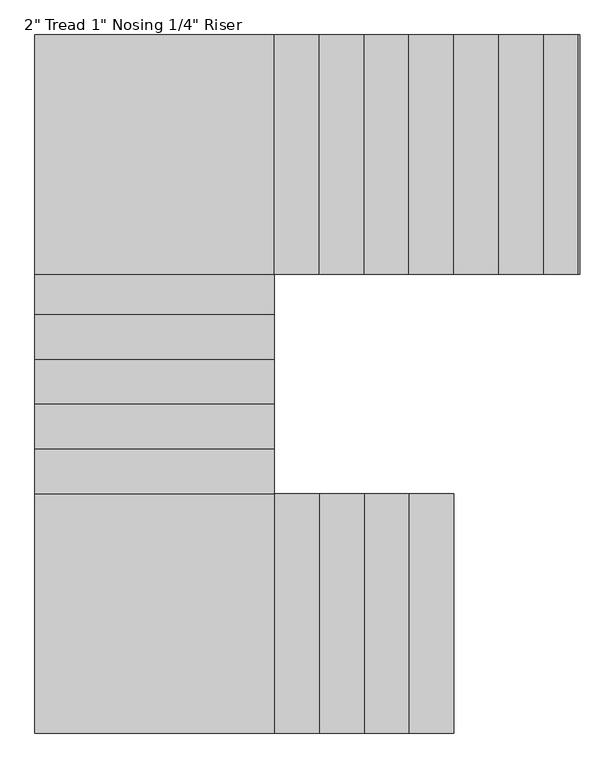
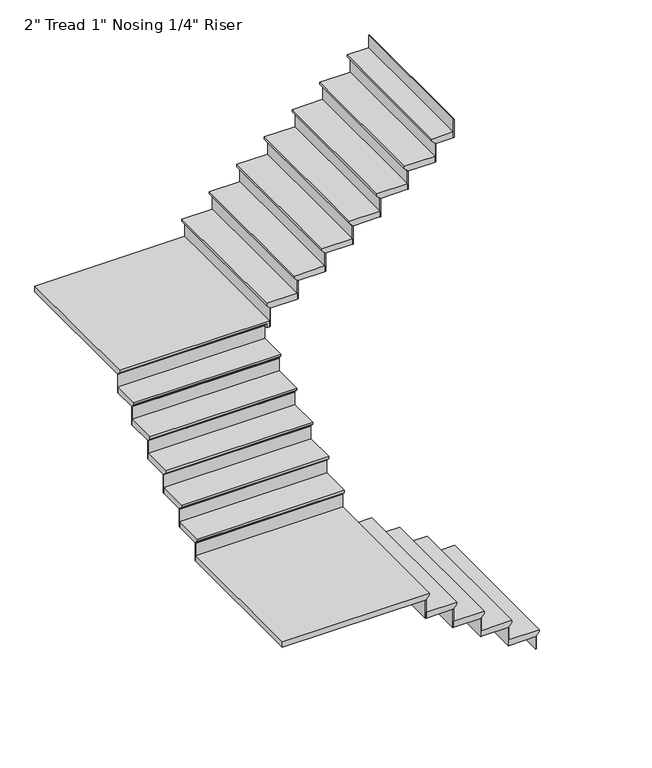
"""IFC4 building model written with IfcOpenShell, lengths in millimetres: stair flight geometry."""

from ifc_helpers import new_model, si_unit, origin, place, context, project, spatial, faceted_brep, source, transform, mapped, element, save


def stair_flight_424eac51(model_context):
    return source(origin(), model_context, "Body", "Brep", [
        faceted_brep([(-2683.1105391, -1521.8373761, 6389.7710526), (-2683.1105391, -1521.8373761, 6408.8210526), (-2683.1105391, -2741.0373761, 6408.8210526), (-2683.1105391, -2741.0373761, 6389.7710526), (-2708.5105391, -1521.8373761, 6364.3710526), (-2708.5105391, -2741.0373761, 6364.3710526), (-2937.1105391, -1521.8373761, 6408.8210526), (-2937.1105391, -2741.0373761, 6408.8210526), (-2708.5105391, -2741.0373761, 6358.0210526), (-2937.1105391, -2741.0373761, 6358.0210526), (-2937.1105391, -1521.8373761, 6358.0210526), (-2708.5105391, -1521.8373761, 6358.0210526)], [[[0, 1, 2, 3]], [[4, 0, 3, 5]], [[2, 1, 6, 7]], [[8, 9, 10, 11]], [[2, 7, 9, 8, 5, 3]], [[8, 11, 4, 5]], [[6, 1, 0, 4, 11, 10]], [[7, 6, 10, 9]]]),
        faceted_brep([(-2708.5105391, -1521.8373761, 6358.0210526), (-2708.5105391, -1521.8373761, 6248.4), (-2714.8605391, -1521.8373761, 6248.4), (-2714.8605391, -1521.8373761, 6358.0210526), (-2708.5105391, -2741.0373761, 6358.0210526), (-2714.8605391, -2741.0373761, 6358.0210526), (-2714.8605391, -2741.0373761, 6248.4), (-2708.5105391, -2741.0373761, 6248.4)], [[[0, 1, 2, 3]], [[4, 5, 6, 7]], [[1, 0, 4, 7]], [[2, 1, 7, 6]], [[3, 2, 6, 5]], [[0, 3, 5, 4]]]),
        faceted_brep([(-2937.1105391, -1521.8373761, 6518.4421053), (-2937.1105391, -1521.8373761, 6358.0210526), (-2943.4605391, -1521.8373761, 6358.0210526), (-2943.4605391, -1521.8373761, 6518.4421053), (-2937.1105391, -2741.0373761, 6518.4421053), (-2943.4605391, -2741.0373761, 6518.4421053), (-2943.4605391, -2741.0373761, 6358.0210526), (-2937.1105391, -2741.0373761, 6358.0210526)], [[[0, 1, 2, 3]], [[4, 5, 6, 7]], [[1, 0, 4, 7]], [[2, 1, 7, 6]], [[3, 2, 6, 5]], [[0, 3, 5, 4]]]),
        faceted_brep([(-2911.7105391, -2741.0373761, 6569.2421053), (-2911.7105391, -1521.8373761, 6569.2421053), (-3165.7105391, -1521.8373761, 6569.2421053), (-3165.7105391, -2741.0373761, 6569.2421053), (-2937.1105391, -2741.0373761, 6518.4421053), (-3165.7105391, -2741.0373761, 6518.4421053), (-3165.7105391, -1521.8373761, 6518.4421053), (-2937.1105391, -1521.8373761, 6518.4421053), (-2937.1105391, -2741.0373761, 6524.7921053), (-2911.7105391, -2741.0373761, 6550.1921053), (-2937.1105391, -1521.8373761, 6524.7921053), (-2911.7105391, -1521.8373761, 6550.1921053)], [[[0, 1, 2, 3]], [[4, 5, 6, 7]], [[0, 3, 5, 4, 8, 9]], [[4, 7, 10, 8]], [[2, 1, 11, 10, 7, 6]], [[3, 2, 6, 5]], [[11, 1, 0, 9]], [[10, 11, 9, 8]]]),
        faceted_brep([(-3165.7105391, -1521.8373761, 6678.8631579), (-3165.7105391, -1521.8373761, 6518.4421053), (-3172.0605391, -1521.8373761, 6518.4421053), (-3172.0605391, -1521.8373761, 6678.8631579), (-3165.7105391, -2741.0373761, 6678.8631579), (-3172.0605391, -2741.0373761, 6678.8631579), (-3172.0605391, -2741.0373761, 6518.4421053), (-3165.7105391, -2741.0373761, 6518.4421053)], [[[0, 1, 2, 3]], [[4, 5, 6, 7]], [[1, 0, 4, 7]], [[2, 1, 7, 6]], [[3, 2, 6, 5]], [[0, 3, 5, 4]]]),
        faceted_brep([(-3140.3105391, -2741.0373761, 6729.6631579), (-3140.3105391, -1521.8373761, 6729.6631579), (-3394.3105391, -1521.8373761, 6729.6631579), (-3394.3105391, -2741.0373761, 6729.6631579), (-3165.7105391, -2741.0373761, 6678.8631579), (-3394.3105391, -2741.0373761, 6678.8631579), (-3394.3105391, -1521.8373761, 6678.8631579), (-3165.7105391, -1521.8373761, 6678.8631579), (-3165.7105391, -2741.0373761, 6685.2131579), (-3140.3105391, -2741.0373761, 6710.6131579), (-3165.7105391, -1521.8373761, 6685.2131579), (-3140.3105391, -1521.8373761, 6710.6131579)], [[[0, 1, 2, 3]], [[4, 5, 6, 7]], [[0, 3, 5, 4, 8, 9]], [[4, 7, 10, 8]], [[2, 1, 11, 10, 7, 6]], [[3, 2, 6, 5]], [[11, 1, 0, 9]], [[10, 11, 9, 8]]]),
        faceted_brep([(-3394.3105391, -1521.8373761, 6839.2842105), (-3394.3105391, -1521.8373761, 6678.8631579), (-3400.6605391, -1521.8373761, 6678.8631579), (-3400.6605391, -1521.8373761, 6839.2842105), (-3394.3105391, -2741.0373761, 6839.2842105), (-3400.6605391, -2741.0373761, 6839.2842105), (-3400.6605391, -2741.0373761, 6678.8631579), (-3394.3105391, -2741.0373761, 6678.8631579)], [[[0, 1, 2, 3]], [[4, 5, 6, 7]], [[1, 0, 4, 7]], [[2, 1, 7, 6]], [[3, 2, 6, 5]], [[0, 3, 5, 4]]]),
        faceted_brep([(-3368.9105391, -2741.0373761, 6890.0842105), (-3368.9105391, -1521.8373761, 6890.0842105), (-3622.9105391, -1521.8373761, 6890.0842105), (-3622.9105391, -2741.0373761, 6890.0842105), (-3394.3105391, -2741.0373761, 6839.2842105), (-3622.9105391, -2741.0373761, 6839.2842105), (-3622.9105391, -1521.8373761, 6839.2842105), (-3394.3105391, -1521.8373761, 6839.2842105), (-3394.3105391, -2741.0373761, 6845.6342105), (-3368.9105391, -2741.0373761, 6871.0342105), (-3394.3105391, -1521.8373761, 6845.6342105), (-3368.9105391, -1521.8373761, 6871.0342105)], [[[0, 1, 2, 3]], [[4, 5, 6, 7]], [[0, 3, 5, 4, 8, 9]], [[4, 7, 10, 8]], [[2, 1, 11, 10, 7, 6]], [[3, 2, 6, 5]], [[11, 1, 0, 9]], [[10, 11, 9, 8]]]),
        faceted_brep([(-3622.9105391, -1521.8373761, 6999.7052632), (-3622.9105391, -1521.8373761, 6839.2842105), (-3629.2605391, -1521.8373761, 6839.2842105), (-3629.2605391, -1521.8373761, 6999.7052632), (-3622.9105391, -2741.0373761, 6999.7052632), (-3629.2605391, -2741.0373761, 6999.7052632), (-3629.2605391, -2741.0373761, 6839.2842105), (-3622.9105391, -2741.0373761, 6839.2842105)], [[[0, 1, 2, 3]], [[4, 5, 6, 7]], [[1, 0, 4, 7]], [[2, 1, 7, 6]], [[3, 2, 6, 5]], [[0, 3, 5, 4]]]),
        faceted_brep([(-4816.7105391, -1496.4373761, 7050.5052632), (-4816.7105391, -2741.0373761, 7050.5052632), (-3597.5105391, -2741.0373761, 7050.5052632), (-3597.5105391, -1496.4373761, 7050.5052632), (-4816.7105391, -2741.0373761, 6999.7052632), (-4816.7105391, -1496.4373761, 6999.7052632), (-3597.5105391, -1496.4373761, 6999.7052632), (-3597.5105391, -1521.8373761, 6999.7052632), (-3622.9105391, -1521.8373761, 6999.7052632), (-3622.9105391, -2741.0373761, 6999.7052632), (-3622.9105391, -2741.0373761, 7006.0552632), (-3597.5105391, -2741.0373761, 7031.4552632), (-3622.9105391, -1521.8373761, 7006.0552632), (-3597.5105391, -1521.8373761, 7031.4552632)], [[[0, 1, 2, 3]], [[4, 5, 6, 7, 8, 9]], [[1, 0, 5, 4]], [[2, 1, 4, 9, 10, 11]], [[9, 8, 12, 10]], [[8, 7, 13, 12]], [[3, 2, 11, 13, 7, 6]], [[0, 3, 6, 5]], [[11, 10, 12, 13]]]),
        faceted_brep([(-3597.5105391, -1496.4373761, 7160.1263158), (-3597.5105391, -1496.4373761, 6999.7052632), (-3597.5105391, -1490.0873761, 6999.7052632), (-3597.5105391, -1490.0873761, 7160.1263158), (-4816.7105391, -1496.4373761, 7160.1263158), (-4816.7105391, -1490.0873761, 7160.1263158), (-4816.7105391, -1490.0873761, 6999.7052632), (-4816.7105391, -1496.4373761, 6999.7052632)], [[[0, 1, 2, 3]], [[4, 5, 6, 7]], [[1, 0, 4, 7]], [[2, 1, 7, 6]], [[3, 2, 6, 5]], [[0, 3, 5, 4]]]),
        faceted_brep([(-4816.7105391, -1521.8373761, 7210.9263158), (-3597.5105391, -1521.8373761, 7210.9263158), (-3597.5105391, -1267.8373761, 7210.9263158), (-4816.7105391, -1267.8373761, 7210.9263158), (-4816.7105391, -1496.4373761, 7160.1263158), (-4816.7105391, -1267.8373761, 7160.1263158), (-3597.5105391, -1267.8373761, 7160.1263158), (-3597.5105391, -1496.4373761, 7160.1263158), (-4816.7105391, -1496.4373761, 7166.4763158), (-4816.7105391, -1521.8373761, 7191.8763158), (-3597.5105391, -1496.4373761, 7166.4763158), (-3597.5105391, -1521.8373761, 7191.8763158)], [[[0, 1, 2, 3]], [[4, 5, 6, 7]], [[0, 3, 5, 4, 8, 9]], [[4, 7, 10, 8]], [[2, 1, 11, 10, 7, 6]], [[3, 2, 6, 5]], [[11, 1, 0, 9]], [[10, 11, 9, 8]]]),
        faceted_brep([(-3597.5105391, -1267.8373761, 7320.5473684), (-3597.5105391, -1267.8373761, 7160.1263158), (-3597.5105391, -1261.4873761, 7160.1263158), (-3597.5105391, -1261.4873761, 7320.5473684), (-4816.7105391, -1267.8373761, 7320.5473684), (-4816.7105391, -1261.4873761, 7320.5473684), (-4816.7105391, -1261.4873761, 7160.1263158), (-4816.7105391, -1267.8373761, 7160.1263158)], [[[0, 1, 2, 3]], [[4, 5, 6, 7]], [[1, 0, 4, 7]], [[2, 1, 7, 6]], [[3, 2, 6, 5]], [[0, 3, 5, 4]]]),
        faceted_brep([(-4816.7105391, -1293.2373761, 7371.3473684), (-3597.5105391, -1293.2373761, 7371.3473684), (-3597.5105391, -1039.2373761, 7371.3473684), (-4816.7105391, -1039.2373761, 7371.3473684), (-4816.7105391, -1267.8373761, 7320.5473684), (-4816.7105391, -1039.2373761, 7320.5473684), (-3597.5105391, -1039.2373761, 7320.5473684), (-3597.5105391, -1267.8373761, 7320.5473684), (-4816.7105391, -1267.8373761, 7326.8973684), (-4816.7105391, -1293.2373761, 7352.2973684), (-3597.5105391, -1267.8373761, 7326.8973684), (-3597.5105391, -1293.2373761, 7352.2973684)], [[[0, 1, 2, 3]], [[4, 5, 6, 7]], [[0, 3, 5, 4, 8, 9]], [[4, 7, 10, 8]], [[2, 1, 11, 10, 7, 6]], [[3, 2, 6, 5]], [[11, 1, 0, 9]], [[10, 11, 9, 8]]]),
        faceted_brep([(-3597.5105391, -1039.2373761, 7480.9684211), (-3597.5105391, -1039.2373761, 7320.5473684), (-3597.5105391, -1032.8873761, 7320.5473684), (-3597.5105391, -1032.8873761, 7480.9684211), (-4816.7105391, -1039.2373761, 7480.9684211), (-4816.7105391, -1032.8873761, 7480.9684211), (-4816.7105391, -1032.8873761, 7320.5473684), (-4816.7105391, -1039.2373761, 7320.5473684)], [[[0, 1, 2, 3]], [[4, 5, 6, 7]], [[1, 0, 4, 7]], [[2, 1, 7, 6]], [[3, 2, 6, 5]], [[0, 3, 5, 4]]]),
        faceted_brep([(-4816.7105391, -1064.6373761, 7531.7684211), (-3597.5105391, -1064.6373761, 7531.7684211), (-3597.5105391, -810.6373761, 7531.7684211), (-4816.7105391, -810.6373761, 7531.7684211), (-4816.7105391, -1039.2373761, 7480.9684211), (-4816.7105391, -810.6373761, 7480.9684211), (-3597.5105391, -810.6373761, 7480.9684211), (-3597.5105391, -1039.2373761, 7480.9684211), (-4816.7105391, -1039.2373761, 7487.3184211), (-4816.7105391, -1064.6373761, 7512.7184211), (-3597.5105391, -1039.2373761, 7487.3184211), (-3597.5105391, -1064.6373761, 7512.7184211)], [[[0, 1, 2, 3]], [[4, 5, 6, 7]], [[0, 3, 5, 4, 8, 9]], [[4, 7, 10, 8]], [[2, 1, 11, 10, 7, 6]], [[3, 2, 6, 5]], [[11, 1, 0, 9]], [[10, 11, 9, 8]]]),
        faceted_brep([(-3597.5105391, -810.6373761, 7641.3894737), (-3597.5105391, -810.6373761, 7480.9684211), (-3597.5105391, -804.2873761, 7480.9684211), (-3597.5105391, -804.2873761, 7641.3894737), (-4816.7105391, -810.6373761, 7641.3894737), (-4816.7105391, -804.2873761, 7641.3894737), (-4816.7105391, -804.2873761, 7480.9684211), (-4816.7105391, -810.6373761, 7480.9684211)], [[[0, 1, 2, 3]], [[4, 5, 6, 7]], [[1, 0, 4, 7]], [[2, 1, 7, 6]], [[3, 2, 6, 5]], [[0, 3, 5, 4]]]),
        faceted_brep([(-4816.7105391, -836.0373761, 7692.1894737), (-3597.5105391, -836.0373761, 7692.1894737), (-3597.5105391, -582.0373761, 7692.1894737), (-4816.7105391, -582.0373761, 7692.1894737), (-4816.7105391, -810.6373761, 7641.3894737), (-4816.7105391, -582.0373761, 7641.3894737), (-3597.5105391, -582.0373761, 7641.3894737), (-3597.5105391, -810.6373761, 7641.3894737), (-4816.7105391, -810.6373761, 7647.7394737), (-4816.7105391, -836.0373761, 7673.1394737), (-3597.5105391, -810.6373761, 7647.7394737), (-3597.5105391, -836.0373761, 7673.1394737)], [[[0, 1, 2, 3]], [[4, 5, 6, 7]], [[0, 3, 5, 4, 8, 9]], [[4, 7, 10, 8]], [[2, 1, 11, 10, 7, 6]], [[3, 2, 6, 5]], [[11, 1, 0, 9]], [[10, 11, 9, 8]]]),
        faceted_brep([(-3597.5105391, -582.0373761, 7801.8105263), (-3597.5105391, -582.0373761, 7641.3894737), (-3597.5105391, -575.6873761, 7641.3894737), (-3597.5105391, -575.6873761, 7801.8105263), (-4816.7105391, -582.0373761, 7801.8105263), (-4816.7105391, -575.6873761, 7801.8105263), (-4816.7105391, -575.6873761, 7641.3894737), (-4816.7105391, -582.0373761, 7641.3894737)], [[[0, 1, 2, 3]], [[4, 5, 6, 7]], [[1, 0, 4, 7]], [[2, 1, 7, 6]], [[3, 2, 6, 5]], [[0, 3, 5, 4]]]),
        faceted_brep([(-4816.7105391, -607.4373761, 7852.6105263), (-3597.5105391, -607.4373761, 7852.6105263), (-3597.5105391, -378.8373761, 7852.6105263), (-4816.7105391, -378.8373761, 7852.6105263), (-4816.7105391, -582.0373761, 7801.8105263), (-4816.7105391, -378.8373761, 7801.8105263), (-3597.5105391, -378.8373761, 7801.8105263), (-3597.5105391, -582.0373761, 7801.8105263), (-4816.7105391, -582.0373761, 7808.1605263), (-4816.7105391, -607.4373761, 7833.5605263), (-3597.5105391, -582.0373761, 7808.1605263), (-3597.5105391, -607.4373761, 7833.5605263)], [[[0, 1, 2, 3]], [[4, 5, 6, 7]], [[0, 3, 5, 4, 8, 9]], [[4, 7, 10, 8]], [[2, 1, 11, 10, 7, 6]], [[3, 2, 6, 5]], [[11, 1, 0, 9]], [[10, 11, 9, 8]]]),
        faceted_brep([(-3597.5105391, -378.8373761, 7962.2315789), (-3597.5105391, -378.8373761, 7801.8105263), (-3597.5105391, -372.4873761, 7801.8105263), (-3597.5105391, -372.4873761, 7962.2315789), (-4816.7105391, -378.8373761, 7962.2315789), (-4816.7105391, -372.4873761, 7962.2315789), (-4816.7105391, -372.4873761, 7801.8105263), (-4816.7105391, -378.8373761, 7801.8105263)], [[[0, 1, 2, 3]], [[4, 5, 6, 7]], [[1, 0, 4, 7]], [[2, 1, 7, 6]], [[3, 2, 6, 5]], [[0, 3, 5, 4]]]),
        faceted_brep([(-3572.1105391, 814.9626239, 8013.0315789), (-4816.7105391, 814.9626239, 8013.0315789), (-4816.7105391, -404.2373761, 8013.0315789), (-3572.1105391, -404.2373761, 8013.0315789), (-4816.7105391, 814.9626239, 7962.2315789), (-3572.1105391, 814.9626239, 7962.2315789), (-3572.1105391, -404.2373761, 7962.2315789), (-3597.5105391, -404.2373761, 7962.2315789), (-3597.5105391, -378.8373761, 7962.2315789), (-4816.7105391, -378.8373761, 7962.2315789), (-4816.7105391, -378.8373761, 7968.5815789), (-4816.7105391, -404.2373761, 7993.9815789), (-3597.5105391, -378.8373761, 7968.5815789), (-3597.5105391, -404.2373761, 7993.9815789)], [[[0, 1, 2, 3]], [[4, 5, 6, 7, 8, 9]], [[1, 0, 5, 4]], [[2, 1, 4, 9, 10, 11]], [[9, 8, 12, 10]], [[8, 7, 13, 12]], [[3, 2, 11, 13, 7, 6]], [[0, 3, 6, 5]], [[11, 10, 12, 13]]]),
        faceted_brep([(-3572.1105391, -404.2373761, 8122.6526316), (-3572.1105391, -404.2373761, 7962.2315789), (-3565.7605391, -404.2373761, 7962.2315789), (-3565.7605391, -404.2373761, 8122.6526316), (-3572.1105391, 814.9626239, 8122.6526316), (-3565.7605391, 814.9626239, 8122.6526316), (-3565.7605391, 814.9626239, 7962.2315789), (-3572.1105391, 814.9626239, 7962.2315789)], [[[0, 1, 2, 3]], [[4, 5, 6, 7]], [[1, 0, 4, 7]], [[2, 1, 7, 6]], [[3, 2, 6, 5]], [[0, 3, 5, 4]]]),
        faceted_brep([(-3597.5105391, 814.9626239, 8173.4526316), (-3597.5105391, -404.2373761, 8173.4526316), (-3343.5105391, -404.2373761, 8173.4526316), (-3343.5105391, 814.9626239, 8173.4526316), (-3572.1105391, 814.9626239, 8122.6526316), (-3343.5105391, 814.9626239, 8122.6526316), (-3343.5105391, -404.2373761, 8122.6526316), (-3572.1105391, -404.2373761, 8122.6526316), (-3572.1105391, 814.9626239, 8129.0026316), (-3597.5105391, 814.9626239, 8154.4026316), (-3572.1105391, -404.2373761, 8129.0026316), (-3597.5105391, -404.2373761, 8154.4026316)], [[[0, 1, 2, 3]], [[4, 5, 6, 7]], [[0, 3, 5, 4, 8, 9]], [[4, 7, 10, 8]], [[2, 1, 11, 10, 7, 6]], [[3, 2, 6, 5]], [[11, 1, 0, 9]], [[10, 11, 9, 8]]]),
        faceted_brep([(-3343.5105391, -404.2373761, 8283.0736842), (-3343.5105391, -404.2373761, 8122.6526316), (-3337.1605391, -404.2373761, 8122.6526316), (-3337.1605391, -404.2373761, 8283.0736842), (-3343.5105391, 814.9626239, 8283.0736842), (-3337.1605391, 814.9626239, 8283.0736842), (-3337.1605391, 814.9626239, 8122.6526316), (-3343.5105391, 814.9626239, 8122.6526316)], [[[0, 1, 2, 3]], [[4, 5, 6, 7]], [[1, 0, 4, 7]], [[2, 1, 7, 6]], [[3, 2, 6, 5]], [[0, 3, 5, 4]]]),
        faceted_brep([(-3368.9105391, 814.9626239, 8333.8736842), (-3368.9105391, -404.2373761, 8333.8736842), (-3114.9105391, -404.2373761, 8333.8736842), (-3114.9105391, 814.9626239, 8333.8736842), (-3343.5105391, 814.9626239, 8283.0736842), (-3114.9105391, 814.9626239, 8283.0736842), (-3114.9105391, -404.2373761, 8283.0736842), (-3343.5105391, -404.2373761, 8283.0736842), (-3343.5105391, 814.9626239, 8289.4236842), (-3368.9105391, 814.9626239, 8314.8236842), (-3343.5105391, -404.2373761, 8289.4236842), (-3368.9105391, -404.2373761, 8314.8236842)], [[[0, 1, 2, 3]], [[4, 5, 6, 7]], [[0, 3, 5, 4, 8, 9]], [[4, 7, 10, 8]], [[2, 1, 11, 10, 7, 6]], [[3, 2, 6, 5]], [[11, 1, 0, 9]], [[10, 11, 9, 8]]]),
        faceted_brep([(-3114.9105391, -404.2373761, 8443.4947368), (-3114.9105391, -404.2373761, 8283.0736842), (-3108.5605391, -404.2373761, 8283.0736842), (-3108.5605391, -404.2373761, 8443.4947368), (-3114.9105391, 814.9626239, 8443.4947368), (-3108.5605391, 814.9626239, 8443.4947368), (-3108.5605391, 814.9626239, 8283.0736842), (-3114.9105391, 814.9626239, 8283.0736842)], [[[0, 1, 2, 3]], [[4, 5, 6, 7]], [[1, 0, 4, 7]], [[2, 1, 7, 6]], [[3, 2, 6, 5]], [[0, 3, 5, 4]]]),
        faceted_brep([(-3140.3105391, 814.9626239, 8494.2947368), (-3140.3105391, -404.2373761, 8494.2947368), (-2886.3105391, -404.2373761, 8494.2947368), (-2886.3105391, 814.9626239, 8494.2947368), (-3114.9105391, 814.9626239, 8443.4947368), (-2886.3105391, 814.9626239, 8443.4947368), (-2886.3105391, -404.2373761, 8443.4947368), (-3114.9105391, -404.2373761, 8443.4947368), (-3114.9105391, 814.9626239, 8449.8447368), (-3140.3105391, 814.9626239, 8475.2447368), (-3114.9105391, -404.2373761, 8449.8447368), (-3140.3105391, -404.2373761, 8475.2447368)], [[[0, 1, 2, 3]], [[4, 5, 6, 7]], [[0, 3, 5, 4, 8, 9]], [[4, 7, 10, 8]], [[2, 1, 11, 10, 7, 6]], [[3, 2, 6, 5]], [[11, 1, 0, 9]], [[10, 11, 9, 8]]]),
        faceted_brep([(-2886.3105391, -404.2373761, 8603.9157895), (-2886.3105391, -404.2373761, 8443.4947368), (-2879.9605391, -404.2373761, 8443.4947368), (-2879.9605391, -404.2373761, 8603.9157895), (-2886.3105391, 814.9626239, 8603.9157895), (-2879.9605391, 814.9626239, 8603.9157895), (-2879.9605391, 814.9626239, 8443.4947368), (-2886.3105391, 814.9626239, 8443.4947368)], [[[0, 1, 2, 3]], [[4, 5, 6, 7]], [[1, 0, 4, 7]], [[2, 1, 7, 6]], [[3, 2, 6, 5]], [[0, 3, 5, 4]]]),
        faceted_brep([(-2911.7105391, 814.9626239, 8654.7157895), (-2911.7105391, -404.2373761, 8654.7157895), (-2657.7105391, -404.2373761, 8654.7157895), (-2657.7105391, 814.9626239, 8654.7157895), (-2886.3105391, 814.9626239, 8603.9157895), (-2657.7105391, 814.9626239, 8603.9157895), (-2657.7105391, -404.2373761, 8603.9157895), (-2886.3105391, -404.2373761, 8603.9157895), (-2886.3105391, 814.9626239, 8610.2657895), (-2911.7105391, 814.9626239, 8635.6657895), (-2886.3105391, -404.2373761, 8610.2657895), (-2911.7105391, -404.2373761, 8635.6657895)], [[[0, 1, 2, 3]], [[4, 5, 6, 7]], [[0, 3, 5, 4, 8, 9]], [[4, 7, 10, 8]], [[2, 1, 11, 10, 7, 6]], [[3, 2, 6, 5]], [[11, 1, 0, 9]], [[10, 11, 9, 8]]]),
        faceted_brep([(-2657.7105391, -404.2373761, 8764.3368421), (-2657.7105391, -404.2373761, 8603.9157895), (-2651.3605391, -404.2373761, 8603.9157895), (-2651.3605391, -404.2373761, 8764.3368421), (-2657.7105391, 814.9626239, 8764.3368421), (-2651.3605391, 814.9626239, 8764.3368421), (-2651.3605391, 814.9626239, 8603.9157895), (-2657.7105391, 814.9626239, 8603.9157895)], [[[0, 1, 2, 3]], [[4, 5, 6, 7]], [[1, 0, 4, 7]], [[2, 1, 7, 6]], [[3, 2, 6, 5]], [[0, 3, 5, 4]]]),
        faceted_brep([(-2683.1105391, 814.9626239, 8815.1368421), (-2683.1105391, -404.2373761, 8815.1368421), (-2429.1105391, -404.2373761, 8815.1368421), (-2429.1105391, 814.9626239, 8815.1368421), (-2657.7105391, 814.9626239, 8764.3368421), (-2429.1105391, 814.9626239, 8764.3368421), (-2429.1105391, -404.2373761, 8764.3368421), (-2657.7105391, -404.2373761, 8764.3368421), (-2657.7105391, 814.9626239, 8770.6868421), (-2683.1105391, 814.9626239, 8796.0868421), (-2657.7105391, -404.2373761, 8770.6868421), (-2683.1105391, -404.2373761, 8796.0868421)], [[[0, 1, 2, 3]], [[4, 5, 6, 7]], [[0, 3, 5, 4, 8, 9]], [[4, 7, 10, 8]], [[2, 1, 11, 10, 7, 6]], [[3, 2, 6, 5]], [[11, 1, 0, 9]], [[10, 11, 9, 8]]]),
        faceted_brep([(-2429.1105391, -404.2373761, 8924.7578947), (-2429.1105391, -404.2373761, 8764.3368421), (-2422.7605391, -404.2373761, 8764.3368421), (-2422.7605391, -404.2373761, 8924.7578947), (-2429.1105391, 814.9626239, 8924.7578947), (-2422.7605391, 814.9626239, 8924.7578947), (-2422.7605391, 814.9626239, 8764.3368421), (-2429.1105391, 814.9626239, 8764.3368421)], [[[0, 1, 2, 3]], [[4, 5, 6, 7]], [[1, 0, 4, 7]], [[2, 1, 7, 6]], [[3, 2, 6, 5]], [[0, 3, 5, 4]]]),
        faceted_brep([(-2454.5105391, 814.9626239, 8975.5578947), (-2454.5105391, -404.2373761, 8975.5578947), (-2200.5105391, -404.2373761, 8975.5578947), (-2200.5105391, 814.9626239, 8975.5578947), (-2429.1105391, 814.9626239, 8924.7578947), (-2200.5105391, 814.9626239, 8924.7578947), (-2200.5105391, -404.2373761, 8924.7578947), (-2429.1105391, -404.2373761, 8924.7578947), (-2429.1105391, 814.9626239, 8931.1078947), (-2454.5105391, 814.9626239, 8956.5078947), (-2429.1105391, -404.2373761, 8931.1078947), (-2454.5105391, -404.2373761, 8956.5078947)], [[[0, 1, 2, 3]], [[4, 5, 6, 7]], [[0, 3, 5, 4, 8, 9]], [[4, 7, 10, 8]], [[2, 1, 11, 10, 7, 6]], [[3, 2, 6, 5]], [[11, 1, 0, 9]], [[10, 11, 9, 8]]]),
        faceted_brep([(-2200.5105391, -404.2373761, 9085.1789474), (-2200.5105391, -404.2373761, 8924.7578947), (-2194.1605391, -404.2373761, 8924.7578947), (-2194.1605391, -404.2373761, 9085.1789474), (-2200.5105391, 814.9626239, 9085.1789474), (-2194.1605391, 814.9626239, 9085.1789474), (-2194.1605391, 814.9626239, 8924.7578947), (-2200.5105391, 814.9626239, 8924.7578947)], [[[0, 1, 2, 3]], [[4, 5, 6, 7]], [[1, 0, 4, 7]], [[2, 1, 7, 6]], [[3, 2, 6, 5]], [[0, 3, 5, 4]]]),
        faceted_brep([(-2048.1105391, -404.2373761, 9245.6), (-2048.1105391, -404.2373761, 9085.1789474), (-2041.7605391, -404.2373761, 9085.1789474), (-2041.7605391, -404.2373761, 9245.6), (-2048.1105391, 814.9626239, 9245.6), (-2041.7605391, 814.9626239, 9245.6), (-2041.7605391, 814.9626239, 9085.1789474), (-2048.1105391, 814.9626239, 9085.1789474)], [[[0, 1, 2, 3]], [[4, 5, 6, 7]], [[1, 0, 4, 7]], [[2, 1, 7, 6]], [[3, 2, 6, 5]], [[0, 3, 5, 4]]]),
        faceted_brep([(-2225.9105391, 814.9626239, 9135.9789474), (-2225.9105391, -404.2373761, 9135.9789474), (-2048.1105391, -404.2373761, 9135.9789474), (-2048.1105391, 814.9626239, 9135.9789474), (-2200.5105391, 814.9626239, 9085.1789474), (-2048.1105391, 814.9626239, 9085.1789474), (-2048.1105391, -404.2373761, 9085.1789474), (-2200.5105391, -404.2373761, 9085.1789474), (-2200.5105391, 814.9626239, 9091.5289474), (-2225.9105391, 814.9626239, 9116.9289474), (-2200.5105391, -404.2373761, 9091.5289474), (-2225.9105391, -404.2373761, 9116.9289474)], [[[0, 1, 2, 3]], [[4, 5, 6, 7]], [[0, 3, 5, 4, 8, 9]], [[4, 7, 10, 8]], [[2, 1, 11, 10, 7, 6]], [[3, 2, 6, 5]], [[11, 1, 0, 9]], [[10, 11, 9, 8]]]),
    ])


if __name__ == "__main__":
    model = new_model("IFC4")
    model_context = context("Model", 3, world=origin())
    ifc_project = project(units=[si_unit("LENGTHUNIT", "METRE", prefix="MILLI")], contexts=[model_context])
    site = spatial("IfcSite", under=ifc_project)
    building = spatial("IfcBuilding", under=site)
    placement = place(None, origin())
    stair_flight_shape = stair_flight_424eac51(model_context)
    element("IfcStairFlight", 1, ObjectType="2\" Tread 1\" Nosing 1/4\" Riser", at=placement, inside=building, context=model_context, shape_type="MappedRepresentation", body=[
        mapped(stair_flight_shape, transform((0.0, 0.0, 0.0), x_axis=(1.0, 0.0, 0.0), y_axis=(0.0, 1.0, 0.0), z_axis=(0.0, 0.0, 1.0))),
    ])
    save(model, "model.ifc")
